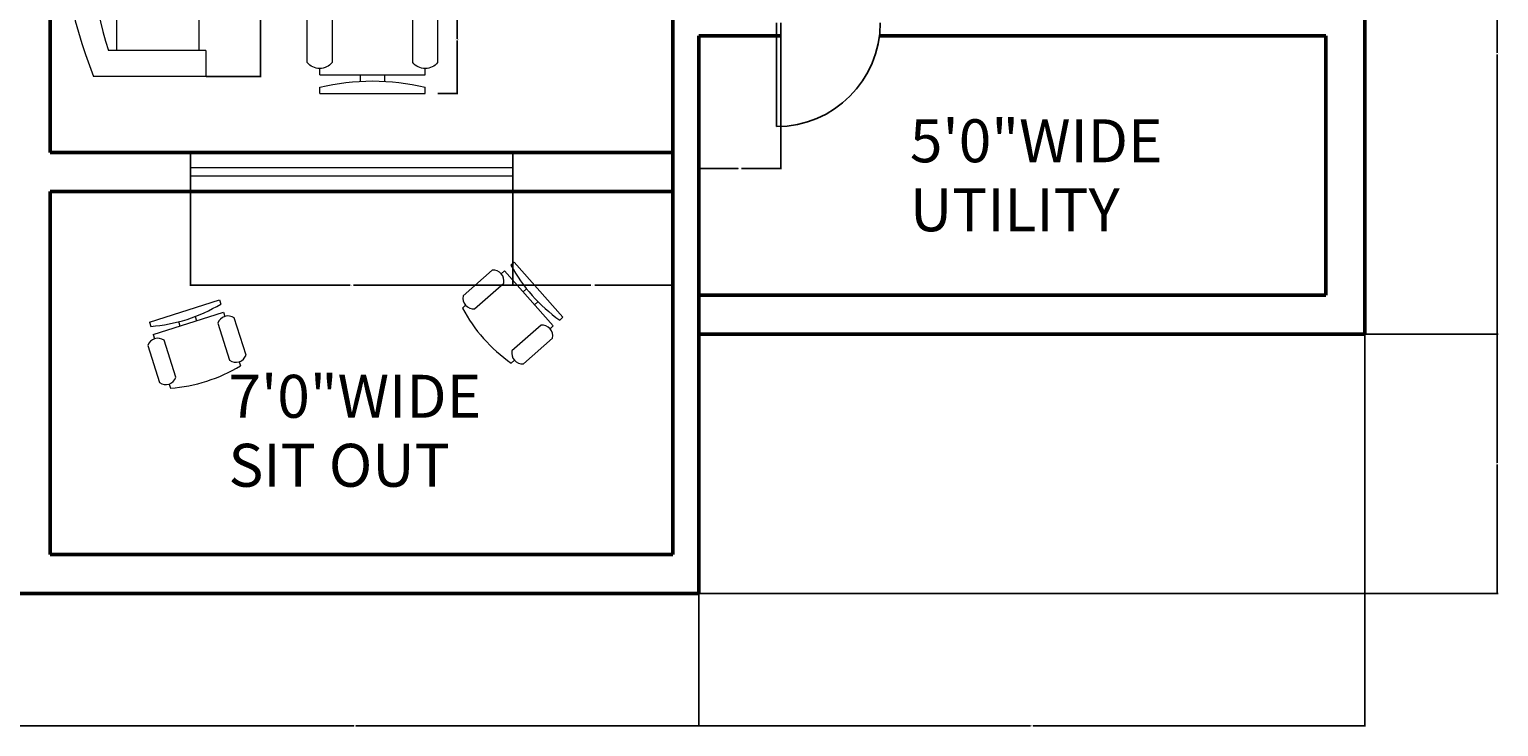
# Model space of a CAD drawing. Units: inches. Extents: x 614 to 1202, y 131 to 752.
# Tile 2 of 5: x 862 to 1202, y 131 to 293. Entities that reach past the tile are written whole.
import ezdxf

# ---------------------------------------------------------------- set-up
doc = ezdxf.new("R2010")
doc.units = ezdxf.units.IN
doc.header["$MEASUREMENT"] = 0
for name, color, linetype, lineweight in [('A-ANNO-DIMS', 2, 'Continuous', 18), ('A-AREA-IDEN', 7, 'Continuous', 18), ('A-DOOR', 3, 'Continuous', 25), ('A-FURN', 8, 'Continuous', 18), ('A-GLAZ', 4, 'Continuous', 18), ('A-WALL', 7, 'Continuous', 50)]:
    doc.layers.add(name, color=color, linetype=linetype, lineweight=lineweight)
doc.styles.get("Standard").update_dxf_attribs({"font": 'arial.ttf'})
doc.dimstyles.get("Standard").update_dxf_attribs({"dimtxt": 0.18, "dimasz": 0.18, "dimexe": 0.18, "dimexo": 0.0625, "dimgap": 0.09, "dimtad": 0, "dimtih": 1, "dimtoh": 1, "dimdec": 0, "dimzin": 0, "dimdsep": 46, "dimlunit": 3, "dimtxsty": 'Standard', "dimcen": 0.09, "dimadec": 0, "dimazin": 0, "dimtfac": 1, "dimtdec": 0, "dimtofl": 0, "dimtmove": 0, "dimatfit": 3, "dimfxl": 1, "dimtolj": 1, "dimtzin": 0, "dimarcsym": 0})

# ---------------------------------------------------------------- blocks, each defined once
blk = doc.blocks.new('Sofa - Roundback 7 ft.')
for p, q in [((-12.00002, -32.4421), (-12.00003, -6.5971)), ((11.99997, -32.4421), (11.99998, -6.5971)), ((-36.000027, -34), (-36.000027, -11.4696)), ((-35.999844, -13.3819), (35.9998, -13.3819)), ((35.99998, -34), (35.99998, -11.4696)), ((-36.000027, -32.4421), (35.99998, -32.4421))]:
    blk.add_line(p, q)
for points in [[(-36.000027, -34), (-42.000027, -34), (-42.000027, -8)], [(41.99998, -8), (41.99998, -34), (35.99998, -34)]]:
    blk.add_lwpolyline(points)
for centre, radius, start, end in [((0, -114.25), 114.25, 68.43141, 111.5686), ((-0.00001, -127.1968), 121.1968, 72.72033, 107.2797)]:
    blk.add_arc(centre, radius, start, end)
blk = doc.blocks.new('Chair - Desk')
for p, q in [((-8.5, 0), (-8.5, -1)), ((-8.5, 0), (8.5, 0)), ((8.5, 0), (8.5, -1)), ((-2, -3), (-2, -1.9355)), ((2, -1.9576), (2, -3)), ((-8.5, -3), (-8.5, -4)), ((-8.5, -3), (8.5, -3)), ((8.5, -3), (8.5, -4)), ((-10.5, -5), (-10.5, -14)), ((-6.5, -14), (-6.5, -5)), ((6.5, -5), (6.5, -14)), ((10.5, -14), (10.5, -5)), ((-8.5, -15), (-8.5, -16)), ((8.5, -15), (8.5, -16))]:
    blk.add_line(p, q)
for centre, radius, start, end in [((0, 34.625), 36.625, 256.5803, 283.4197), ((-8.5, -6.5), 2.5, 36.8699, 143.1301), ((8.5, -6.5), 2.5, 36.8699, 143.1301), ((-8.5, -12.5), 2.5, 216.8699, 323.1301), ((8.5, -12.5), 2.5, 216.8699, 323.1301), ((0, 19.625), 36.625, 256.5803, 283.4197)]:
    blk.add_arc(centre, radius, start, end)
blk = doc.blocks.new('DOOR-SINGLE-24IN')
for p, q in [((0, 0), (0, 24)), ((1, 0), (1, 24))]:
    blk.add_line(p, q)
blk.add_arc((0, 0), 24, 0, 90)
blk = doc.blocks.new('*D14')
at = {"layer": 'A-ANNO-DIMS', "color": 0, "lineweight": -2, "transparency": 16777216}
for p, q in [((956.64, 302.83), (961.28, 302.83)), ((961.1, 302.65), (961.1, 290.57)), ((961.1, 278.13), (961.1, 290.21)), ((956.64, 277.95), (961.28, 277.95))]:
    blk.add_line(p, q, dxfattribs=at)
at = {"layer": 'A-ANNO-DIMS', "color": 0, "transparency": 16777216}
for points in [[(961.07, 302.65), (961.13, 302.65), (961.1, 302.83)], [(961.07, 278.13), (961.13, 278.13), (961.1, 277.95)]]:
    blk.add_solid(points, dxfattribs=at)
at = {"layer": 'Defpoints', "color": 0, "transparency": 16777216}
for p in [(956.58, 302.83), (956.58, 277.95), (961.1, 277.95)]:
    blk.add_point(p, dxfattribs=at)
at = {"layer": 'A-ANNO-DIMS', "color": 0, "transparency": 16777216, "insert": (961.1, 290.39), "char_height": 0.18, "attachment_point": 5}
blk.add_mtext('\\A1;25 TYP.', dxfattribs=at)
blk = doc.blocks.new('*D27')
at = {"layer": 'A-ANNO-DIMS', "color": 0, "lineweight": -2, "transparency": 16777216}
for p, q in [((903.06, 365.86), (915.77, 365.86)), ((915.59, 365.68), (915.59, 324.04)), ((915.59, 282.04), (915.59, 323.68)), ((903.06, 281.86), (915.77, 281.86))]:
    blk.add_line(p, q, dxfattribs=at)
at = {"layer": 'A-ANNO-DIMS', "color": 0, "transparency": 16777216}
for points in [[(915.56, 365.68), (915.62, 365.68), (915.59, 365.86)], [(915.56, 282.04), (915.62, 282.04), (915.59, 281.86)]]:
    blk.add_solid(points, dxfattribs=at)
at = {"layer": 'Defpoints', "color": 0, "transparency": 16777216}
for p in [(902.99, 365.86), (915.59, 365.86), (902.99, 281.86)]:
    blk.add_point(p, dxfattribs=at)
at = {"layer": 'A-ANNO-DIMS', "color": 0, "transparency": 16777216, "insert": (915.59, 323.86), "char_height": 0.18, "attachment_point": 5}
blk.add_mtext('\\A1;SOFA 84 TYP.', dxfattribs=at)
blk = doc.blocks.new('*D60')
at = {"layer": 'A-ANNO-DIMS', "color": 0, "lineweight": -2, "transparency": 16777216}
for p, q in [((1171.06, 351.97), (1201.82, 351.97)), ((1201.64, 351.79), (1201.64, 287.3)), ((1201.64, 222.44), (1201.64, 286.94)), ((1171.06, 222.26), (1201.82, 222.26))]:
    blk.add_line(p, q, dxfattribs=at)
at = {"layer": 'A-ANNO-DIMS', "color": 0, "transparency": 16777216}
for points in [[(1201.61, 351.79), (1201.67, 351.79), (1201.64, 351.97)], [(1201.61, 222.44), (1201.67, 222.44), (1201.64, 222.26)]]:
    blk.add_solid(points, dxfattribs=at)
at = {"layer": 'Defpoints', "color": 0, "transparency": 16777216}
for p in [(1170.99, 351.97), (1201.64, 351.97), (1170.99, 222.26)]:
    blk.add_point(p, dxfattribs=at)
at = {"layer": 'A-ANNO-DIMS', "color": 0, "transparency": 16777216, "insert": (1201.64, 287.12), "char_height": 0.18, "attachment_point": 5}
blk.add_mtext('\\A1;129.7', dxfattribs=at)
blk = doc.blocks.new('*D64')
at = {"layer": 'A-ANNO-DIMS', "color": 0, "lineweight": -2, "transparency": 16777216}
for p, q in [((857.99, 162.2), (857.99, 131.43)), ((1016.99, 162.2), (1016.99, 131.43)), ((858.17, 131.61), (937.21, 131.61)), ((1016.81, 131.61), (937.77, 131.61))]:
    blk.add_line(p, q, dxfattribs=at)
at = {"layer": 'A-ANNO-DIMS', "color": 0, "transparency": 16777216}
for points in [[(858.17, 131.64), (858.17, 131.58), (857.99, 131.61)], [(1016.81, 131.64), (1016.81, 131.58), (1016.99, 131.61)]]:
    blk.add_solid(points, dxfattribs=at)
at = {"layer": 'Defpoints', "color": 0, "transparency": 16777216}
for p in [(857.99, 162.26), (1016.99, 162.26), (1016.99, 131.61)]:
    blk.add_point(p, dxfattribs=at)
at = {"layer": 'A-ANNO-DIMS', "color": 0, "transparency": 16777216, "insert": (937.49, 131.61), "char_height": 0.18, "attachment_point": 5}
blk.add_mtext('\\A1;159', dxfattribs=at)
blk = doc.blocks.new('*D65')
at = {"layer": 'A-ANNO-DIMS', "color": 0, "lineweight": -2, "transparency": 16777216}
for p, q in [((1170.99, 222.2), (1170.99, 131.43)), ((1016.99, 162.2), (1016.99, 131.43)), ((1017.17, 131.61), (1093.71, 131.61)), ((1170.81, 131.61), (1094.27, 131.61))]:
    blk.add_line(p, q, dxfattribs=at)
at = {"layer": 'A-ANNO-DIMS', "color": 0, "transparency": 16777216}
for points in [[(1017.17, 131.64), (1017.17, 131.58), (1016.99, 131.61)], [(1170.81, 131.64), (1170.81, 131.58), (1170.99, 131.61)]]:
    blk.add_solid(points, dxfattribs=at)
at = {"layer": 'Defpoints', "color": 0, "transparency": 16777216}
for p in [(1170.99, 222.26), (1016.99, 162.26), (1170.99, 131.61)]:
    blk.add_point(p, dxfattribs=at)
at = {"layer": 'A-ANNO-DIMS', "color": 0, "transparency": 16777216, "insert": (1093.99, 131.61), "char_height": 0.18, "attachment_point": 5}
blk.add_mtext('\\A1;154', dxfattribs=at)
blk = doc.blocks.new('*D66')
at = {"layer": 'A-ANNO-DIMS', "color": 0, "lineweight": -2, "transparency": 16777216}
for p, q in [((973.98, 264.2), (973.98, 233.43)), ((1010.99, 264.2), (1010.99, 233.43)), ((974.16, 233.61), (992.02, 233.61)), ((1010.81, 233.61), (992.95, 233.61))]:
    blk.add_line(p, q, dxfattribs=at)
at = {"layer": 'A-ANNO-DIMS', "color": 0, "transparency": 16777216}
for points in [[(974.16, 233.64), (974.16, 233.58), (973.98, 233.61)], [(1010.81, 233.64), (1010.81, 233.58), (1010.99, 233.61)]]:
    blk.add_solid(points, dxfattribs=at)
at = {"layer": 'Defpoints', "color": 0, "transparency": 16777216}
for p in [(973.98, 264.26), (1010.99, 264.26), (973.98, 233.61)]:
    blk.add_point(p, dxfattribs=at)
at = {"layer": 'A-ANNO-DIMS', "color": 0, "transparency": 16777216, "insert": (992.49, 233.61), "char_height": 0.18, "attachment_point": 5}
blk.add_mtext('\\A1;37.015', dxfattribs=at)
blk = doc.blocks.new('*D67')
at = {"layer": 'A-ANNO-DIMS', "color": 0, "lineweight": -2, "transparency": 16777216}
for p, q in [((899.43, 264.2), (899.43, 233.43)), ((973.98, 264.2), (973.98, 233.43)), ((899.61, 233.61), (936.31, 233.61)), ((973.8, 233.61), (937.1, 233.61))]:
    blk.add_line(p, q, dxfattribs=at)
at = {"layer": 'A-ANNO-DIMS', "color": 0, "transparency": 16777216}
for points in [[(899.61, 233.64), (899.61, 233.58), (899.43, 233.61)], [(973.8, 233.64), (973.8, 233.58), (973.98, 233.61)]]:
    blk.add_solid(points, dxfattribs=at)
at = {"layer": 'Defpoints', "color": 0, "transparency": 16777216}
for p in [(899.43, 264.26), (973.98, 264.26), (899.43, 233.61)]:
    blk.add_point(p, dxfattribs=at)
at = {"layer": 'A-ANNO-DIMS', "color": 0, "transparency": 16777216, "insert": (936.7, 233.61), "char_height": 0.18, "attachment_point": 5}
blk.add_mtext('\\A1;74.55', dxfattribs=at)
blk = doc.blocks.new('*D69')
at = {"layer": 'A-ANNO-DIMS', "color": 0, "lineweight": -2, "transparency": 16777216}
for p, q in [((1017.06, 222.26), (1201.82, 222.26)), ((1201.64, 222.08), (1201.64, 192.45)), ((1201.64, 162.44), (1201.64, 192.08)), ((1017.06, 162.26), (1201.82, 162.26))]:
    blk.add_line(p, q, dxfattribs=at)
at = {"layer": 'A-ANNO-DIMS', "color": 0, "transparency": 16777216}
for points in [[(1201.61, 222.08), (1201.67, 222.08), (1201.64, 222.26)], [(1201.61, 162.44), (1201.67, 162.44), (1201.64, 162.26)]]:
    blk.add_solid(points, dxfattribs=at)
at = {"layer": 'Defpoints', "color": 0, "transparency": 16777216}
for p in [(1016.99, 222.26), (1201.64, 222.26), (1016.99, 162.26)]:
    blk.add_point(p, dxfattribs=at)
at = {"layer": 'A-ANNO-DIMS', "color": 0, "transparency": 16777216, "insert": (1201.64, 192.26), "char_height": 0.18, "attachment_point": 5}
blk.add_mtext('\\A1;60', dxfattribs=at)
blk = doc.blocks.new('*D80')
at = {"layer": 'A-ANNO-DIMS', "color": 0, "lineweight": -2, "transparency": 16777216}
for p, q in [((1016.99, 291.2), (1016.99, 260.43)), ((1035.95, 291.2), (1035.95, 260.43)), ((1017.17, 260.61), (1026.09, 260.61)), ((1035.77, 260.61), (1026.86, 260.61))]:
    blk.add_line(p, q, dxfattribs=at)
at = {"layer": 'A-ANNO-DIMS', "color": 0, "transparency": 16777216}
for points in [[(1017.17, 260.64), (1017.17, 260.58), (1016.99, 260.61)], [(1035.77, 260.64), (1035.77, 260.58), (1035.95, 260.61)]]:
    blk.add_solid(points, dxfattribs=at)
at = {"layer": 'Defpoints', "color": 0, "transparency": 16777216}
for p in [(1016.99, 291.26), (1035.95, 291.26), (1016.99, 260.61)]:
    blk.add_point(p, dxfattribs=at)
at = {"layer": 'A-ANNO-DIMS', "color": 0, "transparency": 16777216, "insert": (1026.47, 260.61), "char_height": 0.18, "attachment_point": 5}
blk.add_mtext('\\A1;18.96', dxfattribs=at)

msp = doc.modelspace()

# ---------------------------------------------------------------- linework, layer by layer
at = {"layer": 'A-GLAZ'}
for p, q in [((899.4259, 259.7636), (899.4259, 264.2636)), ((899.4259, 264.2636), (899.4259, 255.2636)), ((973.9787, 264.2636), (973.9787, 255.2636)), ((973.9787, 260.7636), (899.4259, 260.7636)), ((973.9787, 258.7636), (899.4259, 258.7636))]:
    msp.add_line(p, q, dxfattribs=at)
at = {"layer": 'A-WALL'}
for p, q in [((1170.9938, 721.2636), (1170.9938, 222.2636)), ((866.9938, 406.2636), (866.9938, 264.2636)), ((1010.9938, 255.2636), (1010.9938, 377.4494)), ((1010.9938, 264.2636), (1010.9938, 377.4494)), ((1010.9938, 231.2636), (1010.9938, 291.2636)), ((1016.9938, 231.2636), (1016.9938, 291.2636)), ((1035.9545, 291.2636), (1016.9938, 291.2636)), ((1161.9938, 291.2636), (1058.7663, 291.2636)), ((1161.9938, 291.2636), (1161.9938, 231.2636)), ((1170.9938, 291.2636), (1170.9938, 231.2636)), ((866.9938, 264.2636), (1010.9938, 264.2636)), ((866.9938, 171.2636), (866.9938, 255.2636)), ((866.9938, 255.2636), (1010.9938, 255.2636)), ((1010.9938, 231.2636), (1010.9938, 255.2636)), ((1010.9938, 255.2636), (1010.9938, 171.2636)), ((1016.9938, 255.2636), (1016.9938, 162.2636)), ((1161.9938, 231.2636), (1016.9938, 231.2636)), ((1170.9938, 222.2636), (1016.9938, 222.2636)), ((1010.9938, 171.2636), (866.9938, 171.2636)), ((1016.9938, 162.2636), (857.9938, 162.2636))]:
    msp.add_line(p, q, dxfattribs=at)

# ---------------------------------------------------------------- block references
at = {"layer": 'A-DOOR', "extrusion": (0, 0, -1), "zscale": -1, "rotation": 180}
msp.add_blockref('DOOR-SINGLE-24IN', (-1034.9549, 294.2632), dxfattribs=at)
at = {"layer": 'A-FURN'}
for name, p, rotation in [('Sofa - Roundback 7 ft.', (868.9942, 323.8607), 90), ('Chair - Desk', (979.9213, 232.5174), 311.5567748077882), ('Chair - Desk', (898.0159, 227.5743), 17.64825068619474)]:
    msp.add_blockref(name, p, dxfattribs=dict(at, rotation=rotation))
at = {"layer": 'A-FURN', "xscale": -1.435269817045705, "yscale": 1.435269817045705, "zscale": 1.435269817045705, "rotation": 180}
msp.add_blockref('Chair - Desk', (941.5074, 277.9487), dxfattribs=at)

# ---------------------------------------------------------------- texts
at = {"layer": 'A-AREA-IDEN'}
for s, p in [('5\'0"WIDE ', (1065.8036, 262.0115)), ('UTILITY', (1065.8036, 246.049)), ('7\'0"WIDE ', (908.2033, 202.8991)), ('SIT OUT', (908.2033, 186.9366))]:
    msp.add_text(s, height=9.93672, dxfattribs=at).set_placement(p)

# ---------------------------------------------------------------- dimensions: what is measured, and where the dimension line sits
at = {"layer": 'A-ANNO-DIMS'}
for base, p1, p2, angle, text, picture, middle in [((915.5942, 365.8607), (902.9942, 281.8607), (902.9942, 365.8607), 90, 'SOFA <> TYP.', '*D27', (915.5942, 323.8607)), ((961.0989, 277.9487), (956.5778, 302.8267), (956.5778, 277.9487), 270, '<> TYP.', '*D14', (961.0989, 290.3877))]:
    dim = msp.add_linear_dim(base=base, p1=p1, p2=p2, angle=angle, text=text, dimstyle='Standard', override={"dimdec": 0, "dimlfac": 1, "dimrnd": 0, "dimzin": 0, "dimdsep": 46, "dimlunit": 2}, dxfattribs=at)
    dim.commit()
    dim.dimension.update_dxf_attribs({"geometry": picture, "text_midpoint": middle})
for base, p1, p2, angle, override, picture, middle in [((1201.6438, 351.971), (1170.9938, 222.2636), (1170.9938, 351.971), 90, {"dimdec": 1, "dimlfac": 1, "dimrnd": 0, "dimzin": 0, "dimdsep": 46, "dimlunit": 2}, '*D60', (1201.6438, 287.1173)), ((1016.9938, 260.6136), (1035.9545, 291.2636), (1016.9938, 291.2636), 180, {"dimdec": 2, "dimlfac": 1, "dimrnd": 0, "dimzin": 0, "dimdsep": 46, "dimlunit": 2}, '*D80', (1026.4741, 260.6136)), ((899.4259, 233.6136), (973.9787, 264.2636), (899.4259, 264.2636), 180, {"dimdec": 2, "dimlfac": 1, "dimrnd": 0, "dimzin": 0, "dimdsep": 46, "dimlunit": 2}, '*D67', (936.7023, 233.6136)), ((973.9787, 233.6136), (1010.9938, 264.2636), (973.9787, 264.2636), 180, {"dimdec": 3, "dimlfac": 1, "dimrnd": 0, "dimzin": 0, "dimdsep": 46, "dimlunit": 2}, '*D66', (992.4862, 233.6136)), ((1201.6438, 222.2636), (1016.9938, 162.2636), (1016.9938, 222.2636), 90, {"dimdec": 0, "dimlfac": 1, "dimrnd": 0, "dimzin": 0, "dimdsep": 46, "dimlunit": 2}, '*D69', (1201.6438, 192.2636))]:
    dim = msp.add_linear_dim(base=base, p1=p1, p2=p2, angle=angle, dimstyle='Standard', override=override, dxfattribs=at)
    dim.commit()
    dim.dimension.update_dxf_attribs({"geometry": picture, "text_midpoint": middle})
for base, p1, p2, picture, middle in [((1170.9938, 131.6136), (1016.9938, 162.2636), (1170.9938, 222.2636), '*D65', (1093.9938, 131.6136)), ((1016.9938, 131.6136), (857.9938, 162.2636), (1016.9938, 162.2636), '*D64', (937.4938, 131.6136))]:
    dim = msp.add_linear_dim(base=base, p1=p1, p2=p2, dimstyle='Standard', override={"dimdec": 0, "dimlfac": 1, "dimrnd": 0, "dimzin": 0, "dimdsep": 46, "dimlunit": 2}, dxfattribs=at)
    dim.commit()
    dim.dimension.update_dxf_attribs({"geometry": picture, "text_midpoint": middle})

doc.saveas('drawing.dxf')
